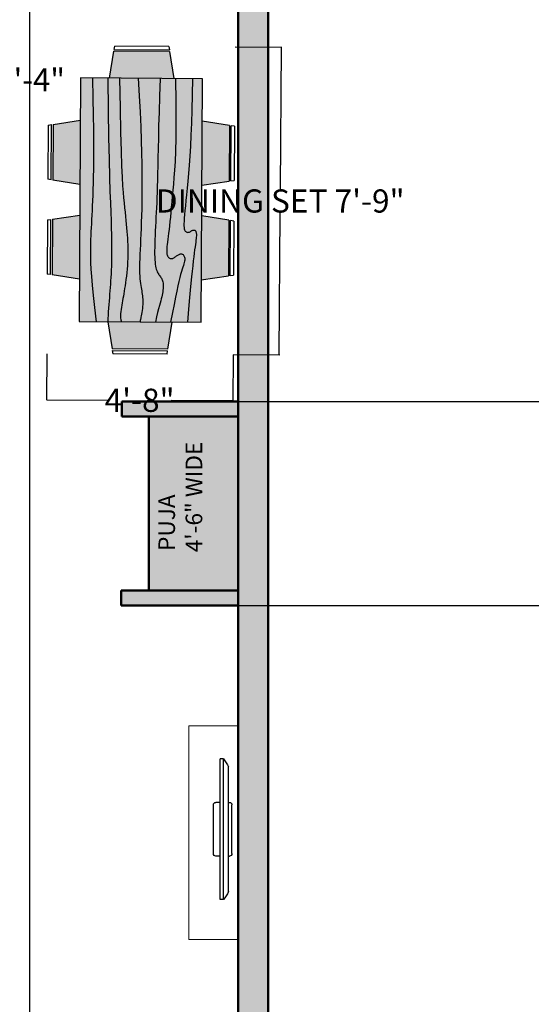
# Model space of a CAD drawing. Units: inches. Extents: x 48 to 822, y -191 to 651.
# Tile 6 of 13: x 291 to 445, y 101 to 398. Entities that reach past the tile are written whole.
import ezdxf

# ---------------------------------------------------------------- set-up
doc = ezdxf.new("R2010")
doc.units = ezdxf.units.IN
doc.header["$MEASUREMENT"] = 0
doc.layers.get('0').update_dxf_attribs({"color": 254})
for name, color, linetype, lineweight in [('A-ANNO-DIMS', 2, 'Continuous', 18), ('A-AREA-IDEN', 7, 'Continuous', 25), ('A-FURN', 8, 'Continuous', 18), ('A-WALL', 7, 'Continuous', 50), ('A-WALL-PATT', 8, 'Continuous', 13)]:
    doc.layers.add(name, color=color, linetype=linetype, lineweight=lineweight)
doc.layers.add('furniture', color=250, linetype='Continuous')
doc.styles.get("Standard").update_dxf_attribs({"font": 'arial.ttf'})
doc.dimstyles.get("Standard").update_dxf_attribs({"dimtxt": 7, "dimasz": 0.18, "dimexe": 0.18, "dimexo": 0.0625, "dimgap": 0.09, "dimtad": 0, "dimtih": 1, "dimtoh": 1, "dimzin": 0, "dimdsep": 46, "dimlunit": 3, "dimtxsty": 'Standard', "dimcen": 0.09, "dimadec": 0, "dimazin": 0, "dimtfac": 1, "dimtofl": 0, "dimtmove": 0, "dimatfit": 3, "dimfxl": 1, "dimtolj": 1, "dimtzin": 0, "dimarcsym": 0})

# ---------------------------------------------------------------- blocks, each defined once
blk = doc.blocks.new('Dining Set - 36 x 72 in.')
for p, q in [((-22, 27.5), (-22.1562, 26.50042)), ((-5.8416, 26.5), (-22.1534, 26.5)), ((-22, 27.5), (-6, 27.5)), ((-5.8437, 26.49966), (-6, 27.5)), ((6, 27.5), (5.8438, 26.50042)), ((22.1584, 26.5), (5.8466, 26.5)), ((6, 27.5), (22, 27.5)), ((22.1563, 26.49966), (22, 27.5)), ((-22.2343, 26.00059), (-23.4847, 17.99762)), ((-22.2304, 26), (-5.7608, 26)), ((-4.5152, 17.99762), (-5.7655, 25.99926)), ((5.7657, 26.00059), (4.5153, 17.99762)), ((5.7696, 26), (22.2392, 26)), ((23.4848, 17.99762), (22.2345, 25.99926)), ((36, 18), (-36, 18)), ((-36, 18), (-36, -18)), ((36, -18), (36, 18)), ((-44.0006, 8.23428), (-35.9976, 9.48474)), ((44.0006, 8.23428), (35.9976, 9.48474)), ((-45.5, 8), (-44.5004, 8.15617)), ((-45.5, 8), (-45.5, -8)), ((-44.5, -8.15843), (-44.5, 8.15338)), ((-44, 8.23041), (-44, -8.23915)), ((44, 8.23041), (44, -8.23915)), ((44.5, -8.15843), (44.5, 8.15338)), ((45.5, 8), (44.5005, 8.15617)), ((45.5, 8), (45.5, -8)), ((-44.4997, -8.15631), (-45.5, -8)), ((-35.9976, -9.48476), (-43.9993, -8.2345)), ((35.9976, -9.48476), (43.9993, -8.2345)), ((44.4997, -8.15631), (45.5, -8)), ((-36, -18), (36, -18)), ((-22.2343, -26.0006), (-23.4847, -17.99762)), ((-4.5152, -17.99762), (-5.7655, -25.99928)), ((5.7657, -26.0006), (4.5153, -17.99762)), ((23.4848, -17.99762), (22.2345, -25.99928)), ((-22.2304, -26), (-5.7608, -26)), ((5.7696, -26), (22.2392, -26)), ((-22, -27.5), (-22.1562, -26.50044)), ((-5.8416, -26.5), (-22.1534, -26.5)), ((-22, -27.5), (-6, -27.5)), ((-5.8437, -26.49967), (-6, -27.5)), ((6, -27.5), (5.8438, -26.50044)), ((22.1584, -26.5), (5.8466, -26.5)), ((6, -27.5), (22, -27.5)), ((22.1563, -26.49967), (22, -27.5))]:
    blk.add_line(p, q)
for points in [[(-36, 15), (-31.1772, 14.97754), (-26.8079, 14.91406), (-22.8538, 14.81543), (-19.276, 14.6875), (-16.0362, 14.53613), (-13.0957, 14.36718), (-10.4159, 14.18652), (-7.9583, 14), (-5.6904, 13.81315), (-3.6035, 13.63021), (-1.6954, 13.45508), (0.0365, 13.29166), (1.5945, 13.14388), (2.9811, 13.01562), (4.1988, 12.9108), (5.25, 12.83333), (6.1393, 12.78613), (6.8802, 12.76823), (7.4883, 12.77767), (7.9792, 12.8125), (8.3685, 12.87077), (8.6719, 12.95052), (8.9049, 13.0498), (9.0833, 13.16666), (9.2205, 13.29899), (9.3216, 13.44401), (9.3895, 13.59879), (9.4271, 13.76041), (9.4373, 13.92594), (9.4232, 14.09245), (9.3875, 14.257), (9.3333, 14.41666), (9.2638, 14.56917), (9.1836, 14.71484), (9.0975, 14.85465), (9.0104, 14.98958), (8.9272, 15.1206), (8.8529, 15.2487), (8.7922, 15.37483), (8.75, 15.5), (8.7305, 15.62467), (8.7344, 15.74739), (8.7617, 15.86621), (8.8125, 15.97916), (8.8867, 16.08431), (8.9844, 16.17968), (9.1055, 16.26334), (9.25, 16.33333), (9.4189, 16.38802), (9.6172, 16.42708), (9.8506, 16.45052), (10.125, 16.45833), (10.4463, 16.45052), (10.8203, 16.42708), (11.2529, 16.38802), (11.75, 16.33333), (12.3184, 16.26318), (12.9694, 16.17838), (13.7151, 16.07991), (14.5677, 15.96875), (15.5395, 15.84586), (16.6426, 15.71224), (17.8893, 15.56884), (19.2917, 15.41666), (20.859, 15.25667), (22.5879, 15.08984), (24.4721, 14.91715), (26.5052, 14.73958), (28.6809, 14.5581), (30.9929, 14.3737), (33.4347, 14.18733), (36, 14)], [(-36, 10), (-28.9766, 10.14274), (-23.1725, 10.20442), (-18.4241, 10.19775), (-14.5677, 10.13541), (-11.4399, 10.03011), (-8.877, 9.89453), (-6.7154, 9.74137), (-4.7917, 9.58333), (-2.9698, 9.43082), (-1.2246, 9.28515), (0.4415, 9.14534), (2.026, 9.01041), (3.5266, 8.87939), (4.9408, 8.7513), (6.266, 8.62516), (7.5, 8.5), (8.6411, 8.37549), (9.6914, 8.2539), (10.6538, 8.13818), (11.5312, 8.03125), (12.3267, 7.93603), (13.043, 7.85547), (13.6831, 7.79248), (14.25, 7.75), (14.7471, 7.7303), (15.1797, 7.73307), (15.5537, 7.75732), (15.875, 7.80208), (16.1494, 7.86637), (16.3828, 7.94922), (16.5811, 8.04964), (16.75, 8.16666), (16.8944, 8.29915), (17.0143, 8.44531), (17.1089, 8.60319), (17.1771, 8.77083), (17.218, 8.94629), (17.2305, 9.1276), (17.2137, 9.31282), (17.1667, 9.5), (17.0895, 9.6875), (16.987, 9.875), (16.8649, 10.0625), (16.7292, 10.25), (16.5856, 10.4375), (16.4401, 10.625), (16.2985, 10.8125), (16.1667, 11), (16.05, 11.18733), (15.9518, 11.3737), (15.8752, 11.5581), (15.8229, 11.73958), (15.798, 11.91715), (15.8034, 12.08984), (15.842, 12.25667), (15.9167, 12.41666), (16.0295, 12.56836), (16.1784, 12.70833), (16.3605, 12.83268), (16.5729, 12.9375), (16.8127, 13.01888), (17.0768, 13.07291), (17.3625, 13.0957), (17.6667, 13.08333), (17.9894, 13.03312), (18.3418, 12.94726), (18.7382, 12.82918), (19.1927, 12.68229), (19.7195, 12.51001), (20.3327, 12.31575), (21.0465, 12.10294), (21.875, 11.875), (22.8357, 11.63354), (23.959, 11.37304), (25.2786, 11.08618), (26.8282, 10.76562), (28.6414, 10.40405), (30.752, 9.99414), (33.1936, 9.52856), (36, 9)], [(-36, 5.5), (-30.7157, 5.3348), (-26.069, 5.20963), (-21.9946, 5.11767), (-18.4271, 5.05208), (-15.3009, 5.00602), (-12.5508, 4.97265), (-10.1112, 4.94515), (-7.9167, 4.91666), (-5.909, 4.88167), (-4.0586, 4.83984), (-2.3429, 4.79215), (-0.7396, 4.73958), (0.7739, 4.6831), (2.22, 4.6237), (3.6213, 4.56233), (5, 4.5), (6.373, 4.43782), (7.7344, 4.3776), (9.0723, 4.32129), (10.375, 4.27083), (11.6309, 4.22819), (12.8281, 4.19531), (13.9551, 4.17415), (15, 4.16666), (15.954, 4.17448), (16.819, 4.19791), (17.6001, 4.23698), (18.3021, 4.29166), (18.9299, 4.36198), (19.4883, 4.44791), (19.9823, 4.54948), (20.4167, 4.66666), (20.7969, 4.79899), (21.1302, 4.94401), (21.4245, 5.09879), (21.6875, 5.26041), (21.9271, 5.42594), (22.1511, 5.59245), (22.3672, 5.757), (22.5834, 5.91666), (22.8065, 6.06868), (23.0404, 6.21093), (23.2879, 6.34147), (23.5521, 6.45833), (23.8358, 6.55957), (24.142, 6.64323), (24.4735, 6.70735), (24.8334, 6.75), (25.2235, 6.76969), (25.642, 6.76692), (26.0858, 6.74267), (26.5521, 6.69791), (27.0379, 6.63362), (27.5404, 6.55078), (28.0565, 6.45036), (28.5834, 6.33333), (29.1242, 6.19987), (29.7071, 6.04687), (30.3661, 5.87044), (31.1354, 5.66666), (32.0493, 5.43164), (33.142, 5.16146), (34.4475, 4.85221), (36, 4.5)], [(-36, -1), (-30.7915, -0.6591), (-26.0195, -0.38216), (-21.6519, -0.16284), (-17.6563, 0.00521), (-14.0005, 0.12833), (-10.6523, 0.21289), (-7.5796, 0.26522), (-4.75, 0.29166), (-2.134, 0.29793), (0.2878, 0.28711), (2.5317, 0.26163), (4.6146, 0.22396), (6.5529, 0.17651), (8.3633, 0.12174), (10.0623, 0.06209), (11.6667, 0), (13.1899, -0.06201), (14.6341, -0.1211), (15.9982, -0.17432), (17.2813, -0.21875), (18.4823, -0.25147), (19.6003, -0.26953), (20.6343, -0.27002), (21.5834, -0.25), (22.4481, -0.20768), (23.2357, -0.14584), (23.9549, -0.06836), (24.6146, 0.02083), (25.2235, 0.11784), (25.7904, 0.21875), (26.3241, 0.31966), (26.8334, 0.41666), (27.3265, 0.50618), (27.8099, 0.58593), (28.2894, 0.65397), (28.7709, 0.70833), (29.2601, 0.74707), (29.763, 0.76823), (30.2855, 0.76985), (30.8334, 0.75), (31.4088, 0.70784), (31.9994, 0.64713), (32.589, 0.57275), (33.1615, 0.48958), (33.7008, 0.4025), (34.1908, 0.3164), (34.6153, 0.23616), (34.9584, 0.16666), (35.2099, 0.11165), (35.3848, 0.07031), (35.504, 0.04069), (35.5886, 0.02083), (35.6594, 0.00879), (35.7377, 0.0026), (35.8442, 0.00032), (36, 0)], [(-36, -6.5), (-27.1843, -6.31267), (-20.084, -6.1263), (-14.469, -5.9419), (-10.1094, -5.76042), (-6.7752, -5.58285), (-4.2363, -5.41016), (-2.2629, -5.24333), (-0.625, -5.08334), (0.8708, -4.93099), (2.2715, -4.78646), (3.5872, -4.64974), (4.8281, -4.52084), (6.0046, -4.39974), (7.127, -4.28646), (8.2053, -4.18099), (9.25, -4.08334), (10.2705, -3.99382), (11.2734, -3.91407), (12.2647, -3.84603), (13.25, -3.79167), (14.2354, -3.75293), (15.2266, -3.73177), (16.2295, -3.73015), (17.25, -3.75), (18.2912, -3.79248), (19.3451, -3.85547), (20.4009, -3.93604), (21.4479, -4.03125), (22.4754, -4.13819), (23.4727, -4.25391), (24.4289, -4.37549), (25.3334, -4.5), (26.1785, -4.62492), (26.9694, -4.74935), (27.7145, -4.87281), (28.4219, -4.99479), (29.1, -5.11483), (29.7572, -5.23242), (30.4016, -5.34709), (31.0417, -5.45834), (31.6837, -5.56437), (32.3262, -5.65821), (32.9658, -5.73153), (33.599, -5.77604), (34.2224, -5.78345), (34.8327, -5.74545), (35.4264, -5.65373), (36, -5.5)], [(-36, -10), (-26.4022, -9.81299), (-18.4675, -9.62891), (-11.9839, -9.45069), (-6.7396, -9.28125), (-2.5226, -9.12354), (0.8789, -8.98047), (3.6769, -8.85498), (6.0833, -8.75), (8.2767, -8.66765), (10.3021, -8.60677), (12.1712, -8.56543), (13.8958, -8.54167), (15.4876, -8.53353), (16.9583, -8.53907), (18.3197, -8.55632), (19.5834, -8.58334), (20.7616, -8.61841), (21.8685, -8.66081), (22.9188, -8.71004), (23.9271, -8.76563), (24.9081, -8.82707), (25.8763, -8.89388), (26.8465, -8.96558), (27.8334, -9.04167), (28.8474, -9.12118), (29.8828, -9.20117), (30.93, -9.27824), (31.9792, -9.34896), (33.0205, -9.40991), (34.0443, -9.45768), (35.0407, -9.48885), (36, -9.5)], [(-36, -14.5), (-30.0881, -14.33513), (-25.0332, -14.21224), (-20.7312, -14.12647), (-17.0781, -14.07292), (-13.97, -14.04671), (-11.3027, -14.04297), (-8.9724, -14.05681), (-6.875, -14.08334), (-4.9224, -14.11833), (-3.0905, -14.16016), (-1.3709, -14.20785), (0.2448, -14.26042), (1.7647, -14.3169), (3.1973, -14.3763), (4.5507, -14.43767), (5.8333, -14.5), (7.0554, -14.5621), (8.235, -14.62175), (9.3922, -14.67652), (10.5469, -14.72396), (11.7192, -14.76164), (12.929, -14.78711), (14.1965, -14.79794), (15.5417, -14.79167), (16.9933, -14.76424), (18.6152, -14.70508), (20.4804, -14.60197), (22.6615, -14.44271), (25.2312, -14.21509), (28.2624, -13.9069), (31.8277, -13.50594), (36, -13)]]:
    blk.add_lwpolyline(points)
blk = doc.blocks.new('dining area')
at = {"layer": 'furniture', "xscale": 0.6659924291999282, "yscale": 0.6659924291999282, "zscale": 0.6659924291999282, "rotation": 90}
blk.add_blockref('Dining Set - 36 x 72 in.', (-0.44, 20.51), dxfattribs=at)
blk = doc.blocks.new('PLASMA-LARGE')
at = {"layer": 'furniture'}
for p, q in [((-7.26, 0), (7.26, 0)), ((-21, -2.5), (21, -2.5)), ((-21, -2.5), (-21, -3.5)), ((-18.61, -1), (18.61, -1)), ((-8, -1), (-8, -0.74)), ((8, -1), (8, -0.74)), ((21, -2.5), (21, -3.5)), ((-21, -3.5), (21, -3.5)), ((-8, -3.5), (-8, -4.76)), ((-7.26, -5.5), (7.26, -5.5)), ((8, -3.5), (8, -4.76))]:
    blk.add_line(p, q, dxfattribs=at)
for centre, radius, start, end in [((-7.26, -0.74), 0.744, 90, 180), ((7.26, -0.74), 0.744, 0, 90), ((-13.97, -11.05), 11.07, 114.7602, 129.4175), ((13.97, -11.05), 11.07, 50.5825, 65.2398), ((-7.26, -4.76), 0.744, 180, 270), ((7.26, -4.76), 0.744, 270, 0)]:
    blk.add_arc(centre, radius, start, end, dxfattribs=at)
blk = doc.blocks.new('TV-UNIT')
for p, q in [((14.9, 64.44), (0, 64.44)), ((0, 64.44), (0, 0)), ((14.9, 64.44), (14.9, 0)), ((0, 0), (14.9, 0))]:
    blk.add_line(p, q)
blk = doc.blocks.new('*D56')
at = {"layer": 'A-ANNO-DIMS', "color": 0, "lineweight": -2, "transparency": 16777216}
for p, q in [((355.49, 390.25), (369.55, 390.16)), ((369.37, 389.98), (369.1, 347.42)), ((368.8, 297.44), (369.06, 340)), ((354.93, 297.35), (368.98, 297.26))]:
    blk.add_line(p, q, dxfattribs=at)
at = {"layer": 'A-ANNO-DIMS', "color": 0, "transparency": 16777216}
for points in [[(369.34, 389.98), (369.4, 389.98), (369.37, 390.16)], [(368.77, 297.44), (368.83, 297.44), (368.8, 297.26)]]:
    blk.add_solid(points, dxfattribs=at)
at = {"layer": 'Defpoints', "color": 0, "transparency": 16777216}
for p in [(355.43, 390.25), (354.86, 297.35), (368.8, 297.26)]:
    blk.add_point(p, dxfattribs=at)
at = {"layer": 'A-ANNO-DIMS', "color": 0, "transparency": 16777216, "insert": (369.08, 343.71), "char_height": 7, "attachment_point": 5}
blk.add_mtext('\\A1;DINING SET 7\'-9"', dxfattribs=at)
blk = doc.blocks.new('*D57')
at = {"layer": 'A-ANNO-DIMS', "color": 0, "lineweight": -2, "transparency": 16777216}
for p, q in [((298.71, 297.63), (298.63, 283.57)), ((354.86, 297.28), (354.78, 283.23)), ((298.81, 283.75), (317.17, 283.64)), ((354.6, 283.41), (336.24, 283.52))]:
    blk.add_line(p, q, dxfattribs=at)
at = {"layer": 'A-ANNO-DIMS', "color": 0, "transparency": 16777216}
for points in [[(298.81, 283.78), (298.81, 283.72), (298.63, 283.75)], [(354.6, 283.44), (354.6, 283.38), (354.78, 283.41)]]:
    blk.add_solid(points, dxfattribs=at)
at = {"layer": 'Defpoints', "color": 0, "transparency": 16777216}
for p in [(298.71, 297.69), (354.86, 297.35), (298.63, 283.75)]:
    blk.add_point(p, dxfattribs=at)
at = {"layer": 'A-ANNO-DIMS', "color": 0, "transparency": 16777216, "insert": (326.7, 283.58), "char_height": 7, "attachment_point": 5}
blk.add_mtext('\\A1;4\'-8"', dxfattribs=at)
blk = doc.blocks.new('*D85')
at = {"layer": 'A-ANNO-DIMS', "color": 0, "lineweight": -2, "transparency": 16777216}
for p, q in [((321.36, 283.18), (790.04, 283.18)), ((789.86, 283), (789.86, 256.14)), ((789.86, 221.87), (789.86, 248.73)), ((321.2, 221.69), (790.04, 221.69))]:
    blk.add_line(p, q, dxfattribs=at)
at = {"layer": 'A-ANNO-DIMS', "color": 0, "transparency": 16777216}
for points in [[(789.83, 283), (789.89, 283), (789.86, 283.18)], [(789.83, 221.87), (789.89, 221.87), (789.86, 221.69)]]:
    blk.add_solid(points, dxfattribs=at)
at = {"layer": 'Defpoints', "color": 0, "transparency": 16777216}
for p in [(321.3, 283.18), (321.14, 221.69), (789.86, 221.69)]:
    blk.add_point(p, dxfattribs=at)
at = {"layer": 'A-ANNO-DIMS', "color": 0, "transparency": 16777216, "insert": (789.86, 252.44), "char_height": 7, "attachment_point": 5}
blk.add_mtext('\\A1;5\'-1 1/2"', dxfattribs=at)
blk = doc.blocks.new('*D92')
at = {"layer": 'A-ANNO-DIMS', "color": 0, "lineweight": -2, "transparency": 16777216}
for p, q in [((275.91, 79.24), (275.91, 641.12)), ((276.09, 640.94), (293.48, 640.94)), ((293.66, 79.24), (293.66, 641.12)), ((293.66, 640.94), (293.84, 640.94))]:
    blk.add_line(p, q, dxfattribs=at)
at = {"layer": 'A-ANNO-DIMS', "color": 0, "transparency": 16777216}
for points in [[(276.09, 640.97), (276.09, 640.91), (275.91, 640.94)], [(293.48, 640.97), (293.48, 640.91), (293.66, 640.94)]]:
    blk.add_solid(points, dxfattribs=at)
at = {"layer": 'Defpoints', "color": 0, "transparency": 16777216}
for p in [(293.66, 640.94), (275.91, 79.18), (293.66, 79.18)]:
    blk.add_point(p, dxfattribs=at)
at = {"layer": 'A-ANNO-DIMS', "color": 0, "transparency": 16777216, "insert": (302.9, 640.94), "char_height": 7, "attachment_point": 5}
blk.add_mtext('\\A1;1\'-6"', dxfattribs=at)

msp = doc.modelspace()

# ---------------------------------------------------------------- hatches: boundary and pattern name
at = {"layer": 'A-FURN'}
h = msp.add_hatch(color=256, dxfattribs=at)
h.dxf.hatch_style = 1
h.paths.add_polyline_path([(317.166, 307.276), (318.392, 299.101), (335.205, 298.998), (336.531, 307.157)])
h.paths.add_polyline_path([(300.494, 338.244), (300.391, 321.432), (308.55, 320.106), (308.669, 339.471)])
h.paths.add_polyline_path([(300.669, 366.829), (300.566, 350.016), (308.725, 348.69), (308.844, 368.055)])
h.paths.add_polyline_path([(318.941, 388.938), (317.615, 380.779), (336.98, 380.661), (335.754, 388.836)])
h.paths.add_polyline_path([(345.595, 367.831), (345.477, 348.466), (353.652, 349.692), (353.755, 366.505)])
h.paths.add_polyline_path([(345.421, 339.246), (345.302, 319.881), (353.477, 321.107), (353.58, 337.92)])
h = msp.add_hatch(color=256, dxfattribs=at)
h.dxf.hatch_style = 1
h.paths.add_polyline_path([(312.495, 380.811), (312.626, 374.774), (312.72, 369.613), (312.781, 365.221), (312.813, 361.491), (312.82, 358.318), (312.807, 355.595), (312.778, 353.216), (312.738, 351.075), (312.69, 349.082), (312.636, 347.212), (312.577, 345.456), (312.513, 343.807), (312.446, 342.256), (312.376, 340.794), (312.305, 339.413), (312.234, 338.104), (312.163, 336.856), (312.094, 335.652), (312.031, 334.471), (311.976, 333.293), (311.93, 332.096), (311.896, 330.861), (311.877, 329.568), (311.875, 328.194), (311.894, 326.712), (311.944, 325.056), (312.038, 323.151), (312.187, 320.924), (312.403, 318.299), (312.699, 315.202), (313.086, 311.56), (313.577, 307.298), (321.233, 307.251), (321.08, 307.837), (320.99, 308.444), (320.955, 309.067), (320.966, 309.704), (321.016, 310.35), (321.095, 311.002), (321.195, 311.658), (321.307, 312.312), (321.424, 312.965), (321.545, 313.622), (321.67, 314.292), (321.796, 314.984), (321.925, 315.705), (322.056, 316.465), (322.188, 317.272), (322.321, 318.134), (322.454, 319.056), (322.584, 320.032), (322.708, 321.049), (322.824, 322.098), (322.927, 323.166), (323.016, 324.243), (323.087, 325.319), (323.137, 326.381), (323.164, 327.423), (323.168, 328.447), (323.153, 329.459), (323.119, 330.465), (323.07, 331.471), (323.007, 332.484), (322.932, 333.508), (322.847, 334.55), (322.753, 335.618), (322.652, 336.719), (322.544, 337.866), (322.427, 339.067), (322.304, 340.335), (322.172, 341.679), (322.033, 343.11), (321.881, 344.701), (320.362, 344.421), (320.408, 344.493), (320.471, 344.442), (321.881, 344.701), (321.734, 346.311), (321.576, 348.327), (321.416, 350.92), (321.255, 354.325), (321.097, 358.776), (320.944, 364.51), (320.798, 371.76), (320.662, 380.761)])
h.paths.add_polyline_path([(308.922, 380.832), (308.472, 307.329), (313.577, 307.298), (313.086, 311.56), (312.699, 315.202), (312.403, 318.299), (312.187, 320.924), (312.038, 323.151), (311.944, 325.056), (311.894, 326.712), (311.875, 328.194), (311.877, 329.568), (311.896, 330.861), (311.93, 332.096), (311.976, 333.293), (312.031, 334.471), (312.094, 335.652), (312.163, 336.856), (312.234, 338.104), (312.305, 339.413), (312.376, 340.794), (312.446, 342.256), (312.513, 343.807), (312.577, 345.456), (312.636, 347.212), (312.69, 349.082), (312.738, 351.075), (312.778, 353.216), (312.807, 355.595), (312.82, 358.318), (312.813, 361.491), (312.781, 365.221), (312.72, 369.613), (312.626, 374.774), (312.495, 380.811)])
h.paths.add_polyline_path([(326.007, 340.78), (325.681, 338.5), (322.757, 335.575), (322.847, 334.55), (322.932, 333.508), (323.007, 332.484), (323.07, 331.471), (323.119, 330.465), (323.153, 329.459), (323.168, 328.447), (323.164, 327.423), (323.137, 326.381), (323.087, 325.319), (323.016, 324.243), (322.927, 323.166), (322.824, 322.098), (322.708, 321.049), (322.584, 320.032), (322.454, 319.056), (322.321, 318.134), (322.188, 317.272), (322.056, 316.465), (321.925, 315.705), (321.796, 314.984), (321.67, 314.292), (321.545, 313.622), (321.424, 312.965), (321.307, 312.312), (321.195, 311.658), (321.095, 311.002), (321.016, 310.35), (320.966, 309.704), (320.955, 309.067), (320.99, 308.444), (321.08, 307.837), (321.233, 307.251), (326.848, 307.216), (326.851, 307.515), (326.875, 307.651), (326.924, 307.844), (326.967, 308.022), (327.025, 308.279), (327.098, 308.629), (327.182, 309.061), (327.273, 309.561), (327.366, 310.111), (327.454, 310.695), (327.534, 311.296), (327.599, 311.899), (327.646, 312.486), (327.67, 313.045), (327.671, 313.579), (327.653, 314.092), (327.616, 314.592), (327.564, 315.084), (327.497, 315.574), (327.419, 316.068), (327.331, 316.572), (327.235, 317.092), (327.135, 317.638), (327.036, 318.217), (326.94, 318.839), (326.854, 319.513), (326.779, 320.248), (326.721, 321.053), (326.683, 321.936), (326.668, 322.905), (326.675, 323.96), (326.701, 325.101), (326.742, 326.327), (326.795, 327.637), (326.858, 329.029), (326.927, 330.503), (327, 332.058), (327.073, 333.695), (327.145, 335.429), (327.212, 337.277), (327.262, 338.905)])
h.paths.add_polyline_path([(320.662, 380.761), (320.798, 371.76), (320.944, 364.51), (321.097, 358.776), (321.255, 354.325), (321.256, 354.318), (324.626, 351.696), (324.66, 351.691), (325.357, 349.598), (327.374, 353.294), (327.357, 354.842), (327.291, 358.26), (327.188, 361.993), (327.042, 366.073), (326.845, 370.533), (326.592, 375.407), (326.277, 380.726)])
h.paths.add_polyline_path([(326.277, 380.726), (326.592, 375.407), (326.845, 370.533), (327.042, 366.073), (327.188, 361.993), (327.291, 358.26), (327.357, 354.842), (327.391, 351.704), (327.4, 348.816), (327.39, 346.145), (331.772, 349.65), (331.741, 349.663), (332.116, 350.938), (332.142, 352.02), (332.184, 354.26), (332.228, 356.75), (332.279, 359.557), (332.345, 362.749), (332.435, 366.39), (332.554, 370.549), (332.711, 375.292), (332.912, 380.686)])
h.paths.add_polyline_path([(332.912, 380.686), (332.711, 375.292), (332.554, 370.549), (332.435, 366.39), (332.345, 362.749), (332.279, 359.557), (332.228, 356.75), (332.184, 354.26), (332.142, 352.02), (332.116, 350.938), (331.741, 349.663), (331.772, 349.65), (327.39, 346.145), (327.364, 343.673), (327.324, 341.382), (327.273, 339.256), (327.212, 337.277), (327.145, 335.429), (327.073, 333.695), (327, 332.058), (326.927, 330.503), (326.858, 329.029), (326.795, 327.637), (326.742, 326.327), (326.701, 325.101), (326.675, 323.96), (326.668, 322.905), (326.683, 321.936), (326.721, 321.053), (326.779, 320.248), (326.854, 319.513), (326.94, 318.839), (327.036, 318.217), (327.135, 317.638), (327.235, 317.092), (327.331, 316.572), (327.419, 316.068), (327.497, 315.574), (327.564, 315.084), (327.616, 314.592), (327.653, 314.092), (327.671, 313.579), (327.67, 313.045), (327.646, 312.486), (327.599, 311.899), (327.534, 311.296), (327.454, 310.695), (327.366, 310.111), (327.273, 309.561), (327.182, 309.061), (327.098, 308.629), (327.025, 308.279), (326.967, 308.022), (326.924, 307.844), (326.893, 307.722), (326.872, 307.636), (326.859, 307.564), (326.852, 307.484), (326.849, 307.375), (326.848, 307.216), (341.141, 307.129), (341.348, 309.747), (341.553, 312.238), (341.756, 314.597), (341.955, 316.817), (342.149, 318.892), (342.337, 320.814), (342.518, 322.578), (342.691, 324.177), (342.855, 325.608), (343.009, 326.88), (343.153, 328.005), (343.284, 328.997), (343.403, 329.866), (343.508, 330.627), (343.599, 331.291), (343.674, 331.871), (343.733, 332.378), (343.775, 332.819), (343.802, 333.201), (343.812, 333.529), (343.805, 333.809), (343.783, 334.048), (343.744, 334.25), (343.69, 334.423), (343.619, 334.571), (343.534, 334.695), (343.438, 334.796), (343.331, 334.872), (343.216, 334.924), (343.095, 334.953), (342.969, 334.958), (342.842, 334.939), (342.714, 334.896), (342.585, 334.835), (342.454, 334.76), (342.319, 334.676), (342.082, 334.525), (341.802, 334.373), (341.482, 334.267), (341.14, 334.24), (340.897, 334.298), (340.739, 334.368), (340.592, 334.472), (340.458, 334.613), (340.34, 334.796), (340.24, 335.034), (340.16, 335.345), (340.103, 335.742), (340.071, 336.244), (340.065, 336.865), (340.088, 337.621), (340.141, 338.528), (340.227, 339.601), (340.342, 340.844), (340.481, 342.258), (340.642, 343.848), (340.82, 345.615), (341.01, 347.562), (341.21, 349.691), (341.415, 352.005), (341.621, 354.513), (341.822, 357.248), (342.013, 360.249), (342.187, 363.555), (342.34, 367.207), (342.466, 371.243), (342.558, 375.703), (342.611, 380.626)])
h.paths.add_polyline_path([(337.06, 350.763), (336.886, 348.8), (336.719, 346.941), (336.56, 345.16), (336.406, 343.46), (336.259, 341.844), (336.121, 340.365), (336.121, 340.365), (335.976, 338.87), (335.839, 337.517), (335.824, 337.378), (335.62, 337.855), (332.056, 339.952), (336.121, 340.365), (336.259, 341.844), (336.406, 343.46), (336.56, 345.16), (336.719, 346.941), (336.886, 348.8), (337.007, 350.166), (335.276, 350.694), (337.096, 351.24)], flags=16)
h.paths.add_polyline_path([(342.611, 380.626), (342.558, 375.703), (342.466, 371.243), (342.34, 367.207), (342.187, 363.555), (342.013, 360.249), (341.822, 357.248), (341.621, 354.513), (341.415, 352.005), (341.21, 349.691), (341.01, 347.562), (340.82, 345.615), (340.642, 343.848), (340.481, 342.258), (340.342, 340.844), (340.227, 339.601), (340.141, 338.528), (340.088, 337.621), (340.065, 336.865), (340.071, 336.244), (340.103, 335.742), (340.16, 335.345), (340.24, 335.034), (340.34, 334.796), (340.458, 334.613), (340.592, 334.472), (340.739, 334.368), (340.897, 334.298), (341.062, 334.258), (341.231, 334.247), (341.401, 334.26), (341.569, 334.296), (341.732, 334.35), (341.888, 334.42), (342.038, 334.501), (342.181, 334.588), (342.432, 334.748), (342.661, 334.879), (342.907, 334.96), (343.158, 334.951), (343.39, 334.845), (343.585, 334.643), (343.69, 334.423), (343.744, 334.25), (343.783, 334.048), (343.805, 333.809), (343.812, 333.529), (343.802, 333.201), (343.775, 332.819), (343.733, 332.378), (343.674, 331.871), (343.599, 331.291), (343.508, 330.627), (343.403, 329.866), (343.284, 328.997), (343.153, 328.005), (343.009, 326.88), (342.855, 325.608), (342.691, 324.177), (342.518, 322.578), (342.337, 320.814), (342.149, 318.892), (341.955, 316.817), (341.756, 314.597), (341.553, 312.238), (341.348, 309.747), (341.141, 307.129), (345.224, 307.104), (345.673, 380.608)])
h.paths.add_polyline_path([(321.256, 354.318), (321.416, 350.92), (321.576, 348.327), (321.734, 346.311), (321.887, 344.638), (322.033, 343.11), (322.172, 341.679), (322.304, 340.335), (322.427, 339.067), (322.544, 337.866), (322.652, 336.719), (322.757, 335.576), (325.681, 338.5), (326.007, 340.78), (327.262, 338.905), (327.273, 339.256), (327.324, 341.382), (327.364, 343.673), (327.39, 346.145), (327.4, 348.816), (327.391, 351.704), (327.374, 353.294), (325.357, 349.598), (324.669, 351.663)])
h.paths.add_polyline_path([(332.056, 339.952), (335.62, 337.855), (335.824, 337.378), (335.839, 337.517), (335.976, 338.87), (336.121, 340.365)], flags=0)
h.paths.add_polyline_path([(335.276, 350.694), (337.007, 350.166), (337.06, 350.763), (337.096, 351.24)], flags=0)
h = msp.add_hatch(color=256, dxfattribs=at)
h.dxf.hatch_style = 1
h.paths.add_polyline_path([(332.912, 380.686), (332.711, 375.292), (332.554, 370.549), (332.435, 366.39), (332.345, 362.749), (332.279, 359.557), (332.228, 356.75), (332.184, 354.26), (332.142, 352.02), (332.093, 349.97), (332.039, 348.081), (331.98, 346.33), (331.916, 344.694), (331.849, 343.149), (331.779, 341.673), (331.708, 340.243), (331.636, 338.836), (331.564, 337.434), (331.494, 336.045), (331.428, 334.679), (331.368, 333.35), (331.317, 332.068), (331.276, 330.846), (331.247, 329.696), (331.233, 328.629), (331.235, 327.655), (331.253, 326.772), (331.288, 325.974), (331.34, 325.257), (331.408, 324.616), (331.492, 324.045), (331.593, 323.54), (331.71, 323.096), (331.842, 322.707), (331.988, 322.366), (332.144, 322.064), (332.308, 321.795), (332.475, 321.549), (332.644, 321.32), (332.81, 321.098), (332.972, 320.876), (333.126, 320.648), (333.27, 320.408), (333.401, 320.154), (333.519, 319.884), (333.621, 319.594), (333.704, 319.281), (333.768, 318.942), (333.809, 318.574), (333.826, 318.176), (333.821, 317.748), (333.794, 317.296), (333.745, 316.82), (333.676, 316.324), (333.589, 315.812), (333.483, 315.285), (333.36, 314.748), (333.22, 314.197), (333.061, 313.603), (332.876, 312.931), (332.664, 312.147), (332.418, 311.216), (332.135, 310.102), (331.811, 308.771), (331.442, 307.188), (336.036, 307.16), (336.593, 310.022), (337.084, 312.512), (337.515, 314.664), (337.896, 316.513), (338.233, 318.092), (338.534, 319.438), (338.807, 320.583), (339.059, 321.562), (339.297, 322.407), (339.519, 323.134), (339.721, 323.759), (339.9, 324.296), (340.053, 324.759), (340.176, 325.163), (340.266, 325.522), (340.319, 325.851), (340.334, 326.161), (340.312, 326.453), (340.259, 326.723), (340.177, 326.968), (340.071, 327.186), (339.946, 327.373), (339.804, 327.525), (339.649, 327.642), (339.487, 327.719), (339.317, 327.759), (339.14, 327.766), (338.959, 327.742), (338.773, 327.689), (338.585, 327.612), (338.394, 327.513), (338.202, 327.395), (338.009, 327.262), (337.817, 327.118), (337.625, 326.971), (337.433, 326.826), (337.24, 326.688), (337.048, 326.565), (336.856, 326.461), (336.664, 326.384), (336.473, 326.337), (336.284, 326.321), (336.099, 326.335), (335.92, 326.378), (335.749, 326.448), (335.588, 326.546), (335.44, 326.669), (335.306, 326.817), (335.187, 326.991), (335.086, 327.194), (335.003, 327.432), (334.939, 327.713), (334.895, 328.041), (334.873, 328.423), (334.873, 328.865), (334.896, 329.372), (334.943, 329.951), (335.011, 330.604), (335.098, 331.335), (335.2, 332.146), (335.315, 333.041), (335.439, 334.023), (335.569, 335.094), (335.704, 336.259), (335.839, 337.517), (335.976, 338.87), (336.116, 340.313), (336.259, 341.844), (336.406, 343.46), (336.56, 345.16), (336.719, 346.941), (336.886, 348.8), (337.06, 350.763), (337.229, 352.969), (337.384, 355.584), (337.511, 358.777), (337.599, 362.713), (337.635, 367.561), (337.608, 373.487), (337.506, 380.658)])
h = msp.add_hatch(color=256, dxfattribs=at)
h.dxf.hatch_style = 1
h.paths.add_polyline_path([(356.451, 283.184), (321.299, 283.184), (321.299, 278.684), (356.451, 278.684)])
h.paths.add_polyline_path([(356.451, 226.187), (321.136, 226.187), (321.136, 221.687), (356.451, 221.687)])
at = {"layer": 'A-WALL-PATT'}
h = msp.add_hatch(color=256, dxfattribs=at)
h.dxf.hatch_style = 1
h.paths.add_polyline_path([(134.451, 590.687), (267.451, 590.687), (267.451, 585.522), (271.951, 585.522), (271.951, 590.687), (356.451, 590.687), (356.451, 83.687), (348.824, 83.687), (348.824, 74.687), (365.451, 74.687), (365.451, 599.687), (125.451, 599.687), (125.451, -67.813), (171.204, -67.813), (171.204, -58.813), (134.451, -58.813), (134.451, 79.187), (193.069, 79.187), (193.069, 83.687), (134.451, 83.687), (134.451, 430.187), (190.775, 430.187), (190.775, 434.687), (134.451, 434.687)])
h.paths.add_polyline_path([(271.951, 550.72), (267.451, 550.72), (267.451, 430.187), (271.951, 430.187)], flags=17)
h.paths.add_polyline_path([(230.951, 432.437), (226.451, 432.437), (226.451, 376.187), (156.909, 376.187), (156.909, 371.687), (164.451, 371.687), (164.451, 359.12), (168.951, 359.12), (168.951, 371.687), (226.451, 371.687), (226.451, 335.687), (230.951, 335.687)], flags=17)
h.paths.add_polyline_path([(168.951, 341.37), (164.451, 341.37), (164.451, 299.687), (134.451, 299.687), (134.451, 295.187), (230.951, 295.187), (230.951, 299.687), (168.951, 299.687)], flags=17)
h.paths.add_polyline_path([(275.909, 83.687), (271.451, 83.687), (245.975, 83.687), (245.975, 79.187), (271.451, 79.187), (271.451, 15.696), (275.951, 15.696), (275.951, 79.177), (275.909, 79.177)], flags=17)
h.paths.add_polyline_path([(275.951, -40.13), (271.451, -40.13), (271.451, -58.813), (227.03, -58.813), (227.03, -67.813), (275.951, -67.813)], flags=17)
h = msp.add_hatch(color=256, dxfattribs=at)
h.dxf.hatch_style = 1
h.paths.add_polyline_path([(153.965, 226.187), (142.862, 226.187), (142.862, 221.687), (153.965, 221.687)])
h.paths.add_polyline_path([(176.172, 226.187), (165.069, 226.187), (165.069, 221.687), (176.172, 221.687)])
h.paths.add_polyline_path([(198.379, 226.187), (187.276, 226.187), (187.276, 221.687), (198.379, 221.687)])
h.paths.add_polyline_path([(220.587, 226.187), (209.483, 226.187), (209.483, 221.687), (220.587, 221.687)])
h.paths.add_polyline_path([(242.794, 226.187), (231.69, 226.187), (231.69, 221.687), (242.794, 221.687)])
h.paths.add_polyline_path([(264.927, 226.187), (253.897, 226.187), (253.897, 221.687), (264.927, 221.687)])
h.paths.add_polyline_path([(356.451, 278.684), (329.451, 278.684), (329.451, 226.187), (356.451, 226.187)])

# ---------------------------------------------------------------- linework, layer by layer
at = {"layer": 'A-WALL'}
for p, q in [((365.451, 599.687), (365.451, -120.313)), ((356.451, 590.687), (356.451, 83.687)), ((321.299, 283.184), (356.451, 283.184)), ((321.299, 283.184), (321.299, 278.684)), ((321.299, 278.684), (356.451, 278.684)), ((329.451, 278.684), (329.451, 226.187)), ((321.136, 226.187), (321.136, 221.687)), ((321.136, 226.187), (356.451, 226.187)), ((321.136, 221.687), (356.451, 221.687))]:
    msp.add_line(p, q, dxfattribs=at)

# ---------------------------------------------------------------- block references
at = {"layer": 'A-FURN'}
for name, p, xscale, yscale, zscale, rotation in [('dining area', (326.592, 375.407), 1.532904782576659, 1.532904782576659, 1.532904782576659, 179.6497047161238), ('PLASMA-LARGE', (354.501, 154.164), -1.011294184530666, 1.011294184530666, 1.011294184530666, 270)]:
    msp.add_blockref(name, p, dxfattribs=dict(at, xscale=xscale, yscale=yscale, zscale=zscale, rotation=rotation))
msp.add_blockref('TV-UNIT', (341.554, 120.903), dxfattribs=at)

# ---------------------------------------------------------------- texts
at = {"layer": 'A-AREA-IDEN'}
msp.add_text('10\'-5"X11\'-4"', height=6.86603, dxfattribs=at).set_placement((247.07, 376.833))
for s, p in [('4\'-6" WIDE', (345.576, 237.729)), ('PUJA', (337.372, 238.134))]:
    msp.add_text(s, height=5.0075, rotation=90, dxfattribs=at).set_placement(p)

# ---------------------------------------------------------------- dimensions: what is measured, and where the dimension line sits
at = {"layer": 'A-ANNO-DIMS'}
dim = msp.add_linear_dim(base=(293.6592, 640.9365), p1=(275.9088, 79.1772), p2=(293.6592, 79.1772), dimstyle='Standard', override={"dimdec": 1, "dimlfac": 1, "dimrnd": 0, "dimzin": 1, "dimdsep": 46, "dimlunit": 4, "dimfrac": 2}, dxfattribs=at)
dim.commit()
dim.dimension.update_dxf_attribs({"geometry": '*D92', "text_midpoint": (302.9036, 640.9365)})
dim = msp.add_linear_dim(base=(368.798, 297.261), p1=(355.431, 390.247), p2=(354.863, 297.346), angle=269.6497, text='DINING SET <>', dimstyle='Standard', override={"dimdec": 1, "dimlfac": 1, "dimrnd": 0, "dimzin": 1, "dimdsep": 46, "dimlunit": 4, "dimfrac": 2}, dxfattribs=at)
dim.commit()
dim.dimension.update_dxf_attribs({"geometry": '*D56', "text_midpoint": (369.082, 343.711)})
for base, p1, p2, angle, picture, middle in [((298.629, 283.755), (354.863, 297.346), (298.715, 297.69), 179.6497, '*D57', (326.704, 283.583)), ((789.86, 221.687), (321.299, 283.184), (321.136, 221.687), 90, '*D85', (789.86, 252.435))]:
    dim = msp.add_linear_dim(base=base, p1=p1, p2=p2, angle=angle, dimstyle='Standard', override={"dimdec": 1, "dimlfac": 1, "dimrnd": 0, "dimzin": 1, "dimdsep": 46, "dimlunit": 4, "dimfrac": 2}, dxfattribs=at)
    dim.commit()
    dim.dimension.update_dxf_attribs({"geometry": picture, "text_midpoint": middle})

doc.saveas('drawing.dxf')
